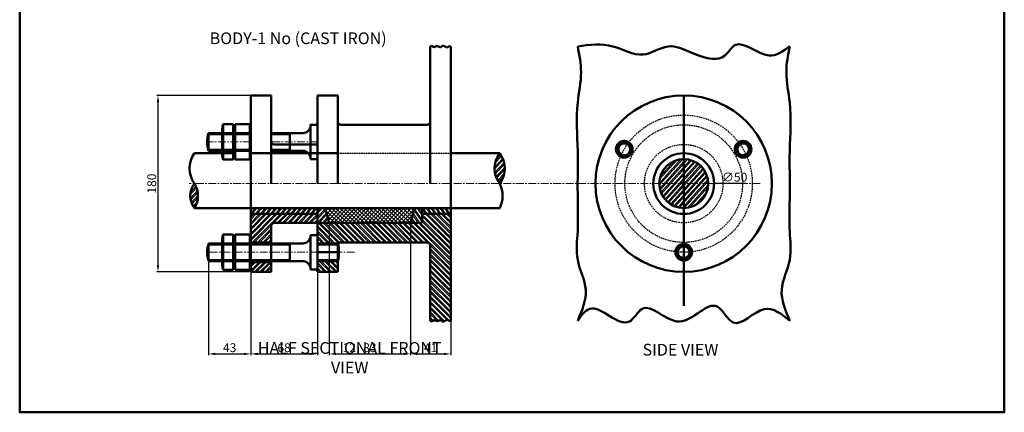
# Model space of a CAD drawing. Units: millimetres. Extents: x -98 to 907, y -783 to 313.
# Tile 1 of 3: x -98 to 907, y -783 to -383. Entities that reach past the tile are written whole.
import ezdxf

# ---------------------------------------------------------------- set-up
doc = ezdxf.new("R2010")
doc.units = ezdxf.units.MM
doc.header["$LTSCALE"] = 0.5
doc.linetypes.add('CENTER', pattern=[50.8, 31.75, -6.35, 6.35, -6.35])
doc.linetypes.add('HIDDEN', pattern=[9.525, 6.35, -3.175])
for name, color, linetype, lineweight in [('M-CNTR', 1, 'CENTER', 18), ('M-DIMS', 2, 'Continuous', 25), ('M-HATC', 8, 'Continuous', 18), ('M-HIDN', 4, 'HIDDEN', 25), ('M-OUTL', 7, 'Continuous', 50), ('M-TEXT', 3, 'Continuous', 25)]:
    doc.layers.add(name, color=color, linetype=linetype, lineweight=lineweight)
doc.styles.get("Standard").update_dxf_attribs({"font": 'arial.ttf'})
doc.dimstyles.new('ISO-25', dxfattribs={"dimtxt": 9, "dimasz": 7, "dimexe": 1.25, "dimexo": 0.625, "dimtad": 1, "dimtoh": 1, "dimtxsty": 'Standard', "dimcen": 2.5, "dimadec": 0, "dimazin": 0, "dimtfac": 1, "dimtofl": 0, "dimtmove": 0, "dimatfit": 3, "dimfxl": 1, "dimarcsym": 0})
pattern_1 = [(228, (1051.4906, -935.3726), (2.831382, -2.549388), []), (228, (1049.697, -935.4666), (2.831382, -2.549388), [])]

# ---------------------------------------------------------------- blocks, each defined once
blk = doc.blocks.new('NUT-HEX')
at = {"ltscale": 0.5}
for p, q in [((0, 16), (36, 16)), ((0, 8.5), (0, 16)), ((9, 8.5), (9, 17)), ((27, 17), (27, 8.5)), ((36, 16), (36, 8.5)), ((0, 1), (0, 8.5)), ((36, 1), (0, 1)), ((9, 1), (9, 8.5)), ((27, 8.5), (27, 1)), ((36, 8.5), (36, 1))]:
    blk.add_line(p, q, dxfattribs=at)
for centre, radius, start, end in [((4.5, 6.4), 10.6, 64.8152, 115.1848), ((18, -24), 41, 77.3196, 102.6804), ((31.5, 6.5), 10.6, 64.7565, 115.2435), ((4.5, 10.6), 10.6, 244.8152, 295.1848), ((18, 41), 41, 257.3196, 282.6804), ((31.5, 10.6), 10.6, 244.7565, 295.2435)]:
    blk.add_arc(centre, radius, start, end, dxfattribs=at)
blk = doc.blocks.new('STUD')
at = {"ltscale": 0.5}
for p, q in [((595.5, 113.7), (595.5, 78.7)), ((602.5, 113.7), (595.5, 113.7)), ((602.5, 78.7), (602.5, 113.7)), ((491.5, 105.2), (587.5, 105.2)), ((491.5, 87.2), (491.5, 105.2)), ((587.5, 87.2), (491.5, 87.2)), ((595.5, 78.7), (602.5, 78.7))]:
    blk.add_line(p, q, dxfattribs=at)
for centre, radius, start, end in [((587.5, 113.2), 8, 270, 0), ((517.6, 96.2), 27.6, 160.9887, 199.0113), ((587.5, 79.2), 8, 0, 90)]:
    blk.add_arc(centre, radius, start, end, dxfattribs=at)
blk = doc.blocks.new('*D41')
at = {"layer": 'Defpoints', "color": 0, "ltscale": 0.5, "transparency": 16777216}
for p in [(137.7, -639.8), (205.7, -639.8), (205.7, -723.6)]:
    blk.add_point(p, dxfattribs=at)
at = {"layer": 'M-DIMS', "color": 0, "lineweight": -2, "ltscale": 0.5, "transparency": 16777216}
for p, q in [((137.7, -640.5), (137.7, -724.8)), ((205.7, -640.5), (205.7, -724.8)), ((144.7, -723.6), (198.7, -723.6))]:
    blk.add_line(p, q, dxfattribs=at)
at = {"layer": 'M-DIMS', "color": 0, "ltscale": 0.5, "transparency": 16777216}
for points in [[(144.7, -722.4), (144.7, -724.8), (137.7, -723.6)], [(198.7, -722.4), (198.7, -724.8), (205.7, -723.6)]]:
    blk.add_solid(points, dxfattribs=at)
at = {"layer": 'M-DIMS', "color": 0, "ltscale": 0.5, "transparency": 16777216, "insert": (171.7, -718.4), "char_height": 9, "attachment_point": 5}
blk.add_mtext('68', dxfattribs=at)
blk = doc.blocks.new('*D42')
at = {"layer": 'Defpoints', "color": 0, "ltscale": 0.5, "transparency": 16777216}
for p in [(205.7, -589.8), (217.7, -589.8), (217.7, -723.6)]:
    blk.add_point(p, dxfattribs=at)
at = {"layer": 'M-DIMS', "color": 0, "lineweight": -2, "ltscale": 0.5, "transparency": 16777216}
for p, q in [((205.7, -590.5), (205.7, -724.8)), ((217.7, -590.5), (217.7, -724.8)), ((198.7, -723.6), (191.7, -723.6)), ((224.7, -723.6), (244.9, -723.6))]:
    blk.add_line(p, q, dxfattribs=at)
at = {"layer": 'M-DIMS', "color": 0, "ltscale": 0.5, "transparency": 16777216}
for points in [[(198.7, -722.4), (198.7, -724.8), (205.7, -723.6)], [(224.7, -722.4), (224.7, -724.8), (217.7, -723.6)]]:
    blk.add_solid(points, dxfattribs=at)
at = {"layer": 'M-DIMS', "color": 0, "ltscale": 0.5, "transparency": 16777216, "insert": (238.3, -718.4), "char_height": 9, "attachment_point": 5}
blk.add_mtext('12', dxfattribs=at)
blk = doc.blocks.new('*D43')
at = {"layer": 'Defpoints', "color": 0, "ltscale": 0.5, "transparency": 16777216}
for p in [(217.7, -589.8), (300.7, -589.8), (300.7, -723.6)]:
    blk.add_point(p, dxfattribs=at)
at = {"layer": 'M-DIMS', "color": 0, "lineweight": -2, "ltscale": 0.5, "transparency": 16777216}
for p, q in [((217.7, -590.5), (217.7, -724.8)), ((300.7, -590.5), (300.7, -724.8)), ((224.7, -723.6), (293.7, -723.6))]:
    blk.add_line(p, q, dxfattribs=at)
at = {"layer": 'M-DIMS', "color": 0, "ltscale": 0.5, "transparency": 16777216}
for points in [[(224.7, -722.4), (224.7, -724.8), (217.7, -723.6)], [(293.7, -722.4), (293.7, -724.8), (300.7, -723.6)]]:
    blk.add_solid(points, dxfattribs=at)
at = {"layer": 'M-DIMS', "color": 0, "ltscale": 0.5, "transparency": 16777216, "insert": (259.2, -718.4), "char_height": 9, "attachment_point": 5}
blk.add_mtext('83', dxfattribs=at)
blk = doc.blocks.new('*D44')
at = {"layer": 'Defpoints', "color": 0, "ltscale": 0.5, "transparency": 16777216}
for p in [(341.7, -580.8), (300.7, -589.8), (341.7, -723.6)]:
    blk.add_point(p, dxfattribs=at)
at = {"layer": 'M-DIMS', "color": 0, "lineweight": -2, "ltscale": 0.5, "transparency": 16777216}
for p, q in [((341.7, -581.5), (341.7, -724.8)), ((300.7, -590.5), (300.7, -724.8)), ((307.7, -723.6), (334.7, -723.6))]:
    blk.add_line(p, q, dxfattribs=at)
at = {"layer": 'M-DIMS', "color": 0, "ltscale": 0.5, "transparency": 16777216}
for points in [[(307.7, -722.4), (307.7, -724.8), (300.7, -723.6)], [(334.7, -722.4), (334.7, -724.8), (341.7, -723.6)]]:
    blk.add_solid(points, dxfattribs=at)
at = {"layer": 'M-DIMS', "color": 0, "ltscale": 0.5, "transparency": 16777216, "insert": (321.2, -718.4), "char_height": 9, "attachment_point": 5}
blk.add_mtext('41', dxfattribs=at)
blk = doc.blocks.new('*D45')
at = {"layer": 'Defpoints', "color": 0, "ltscale": 0.5, "transparency": 16777216}
for p in [(94.7, -628.8), (137.7, -639.8), (137.7, -723.6)]:
    blk.add_point(p, dxfattribs=at)
at = {"layer": 'M-DIMS', "color": 0, "lineweight": -2, "ltscale": 0.5, "transparency": 16777216}
for p, q in [((94.7, -629.5), (94.7, -724.8)), ((137.7, -640.5), (137.7, -724.8)), ((101.7, -723.6), (130.7, -723.6))]:
    blk.add_line(p, q, dxfattribs=at)
at = {"layer": 'M-DIMS', "color": 0, "ltscale": 0.5, "transparency": 16777216}
for points in [[(101.7, -722.4), (101.7, -724.8), (94.7, -723.6)], [(130.7, -722.4), (130.7, -724.8), (137.7, -723.6)]]:
    blk.add_solid(points, dxfattribs=at)
at = {"layer": 'M-DIMS', "color": 0, "ltscale": 0.5, "transparency": 16777216, "insert": (116.2, -718.4), "char_height": 9, "attachment_point": 5}
blk.add_mtext('43', dxfattribs=at)
blk = doc.blocks.new('*D46')
at = {"layer": 'Defpoints', "color": 0, "ltscale": 0.5, "transparency": 16777216}
for p in [(137.7, -459.8), (43, -639.8), (137.7, -639.8)]:
    blk.add_point(p, dxfattribs=at)
at = {"layer": 'M-DIMS', "color": 0, "lineweight": -2, "ltscale": 0.5, "transparency": 16777216}
for p, q in [((137, -459.8), (41.7, -459.8)), ((43, -466.8), (43, -632.8)), ((137, -639.8), (41.7, -639.8))]:
    blk.add_line(p, q, dxfattribs=at)
at = {"layer": 'M-DIMS', "color": 0, "ltscale": 0.5, "transparency": 16777216}
for points in [[(41.8, -466.8), (44.2, -466.8), (43, -459.8)], [(41.8, -632.8), (44.2, -632.8), (43, -639.8)]]:
    blk.add_solid(points, dxfattribs=at)
at = {"layer": 'M-DIMS', "color": 0, "ltscale": 0.5, "transparency": 16777216, "insert": (37.8, -549.8), "char_height": 9, "attachment_point": 5, "rotation": 90}
blk.add_mtext('180', dxfattribs=at)
blk = doc.blocks.new('*D54')
at = {"layer": 'Defpoints', "color": 0, "ltscale": 0.5, "transparency": 16777216}
for p in [(554.5, -549.8), (604.5, -549.8)]:
    blk.add_point(p, dxfattribs=at)
at = {"layer": 'M-DIMS', "color": 0, "lineweight": -2, "ltscale": 0.5, "transparency": 16777216}
for p, q in [((577, -549.8), (582, -549.8)), ((579.5, -552.3), (579.5, -547.3)), ((619.5, -549.8), (611.5, -549.8)), ((642.7, -549.8), (619.5, -549.8))]:
    blk.add_line(p, q, dxfattribs=at)
at = {"layer": 'M-DIMS', "color": 0, "ltscale": 0.5, "transparency": 16777216}
blk.add_solid([(611.5, -548.7), (611.5, -551), (604.5, -549.8)], dxfattribs=at)
at = {"layer": 'M-DIMS', "color": 0, "ltscale": 0.5, "transparency": 16777216, "insert": (631.4, -544.4), "char_height": 9, "attachment_point": 5}
blk.add_mtext('∅50', dxfattribs=at)

msp = doc.modelspace()

# ---------------------------------------------------------------- hatches: boundary and pattern name
at = {"layer": 'M-HATC', "ltscale": 0.5}
h = msp.add_hatch(dxfattribs=at)
h.set_pattern_fill('ANSI32', color=256, scale=0.4, angle=363)
h.set_pattern_definition([(48, (783.4996, -819.342), (-2.831382, 2.549388), []), (48, (785.293, -819.248), (-2.831382, 2.549388), [])])
h.paths.add_polyline_path([(137.6706, -580.8393), (205.6706, -580.8393), (205.6706, -589.8393), (217.6706, -589.8393), (213.6514, -574.8393), (137.6706, -574.8393)])
edge = h.paths.add_edge_path()
edge.add_arc((127.101, -520.8393), 10.5748, 358.1956679, 361.8043321)
edge.add_line((137.6706, -520.5063), (137.6706, -521.1722))
h = msp.add_hatch(dxfattribs=at)
h.set_pattern_fill('ANSI32', color=256, scale=0.4, angle=183)
h.set_pattern_definition(pattern_1)
h.paths.add_polyline_path([(391.6706, -518.8393, 0.336981318), (391.6706, -549.8393, 0.336981318)])
h = msp.add_hatch(dxfattribs=at)
h.set_pattern_fill('ANSI32', color=256, scale=0.4, angle=183)
h.paths.add_polyline_path([(579.4617, -524.8393, 0.414213562), (554.4617, -549.8393), (579.4617, -549.8393)])
h.paths.add_polyline_path([(579.4617, -524.8393), (579.4617, -549.8393), (604.4617, -549.8393, 0.414213562)])
h.paths.add_polyline_path([(604.4617, -549.8393), (579.4617, -549.8393), (579.4617, -574.8393, 0.414213562)])
h.paths.add_polyline_path([(579.4617, -549.8393), (554.4617, -549.8393, 0.414213562), (579.4617, -574.8393)])
h = msp.add_hatch(dxfattribs=at)
h.set_pattern_fill('ANSI32', color=256, scale=0.4, angle=183)
h.set_pattern_definition(pattern_1)
h.paths.add_polyline_path([(80.2178, -574.8393, 0.290271984), (80.2178, -549.8393, 0.335154212)])
h = msp.add_hatch(dxfattribs=at)
h.set_pattern_fill('ANSI32', color=256, scale=0.4)
h.set_pattern_definition([(45, (37.2156, -636.4595), (-2.69408, 2.69408), []), (45, (39.0116, -636.4595), (-2.69408, 2.69408), [])])
h.paths.add_polyline_path([(137.6706, -629.8393), (137.6706, -639.8393), (158.6706, -639.8393), (158.6706, -629.8393)])
h.paths.add_polyline_path([(137.6706, -609.8393), (158.6706, -609.8393), (158.6706, -592.8393, -0.414213562), (161.6706, -589.8393), (205.6706, -589.8393), (205.6706, -580.8393), (137.6706, -580.8393)])
h = msp.add_hatch(dxfattribs=at)
h.set_pattern_fill('ANSI32', color=256, scale=0.4, angle=90)
h.set_pattern_definition([(135, (72.0148, -304.6603), (-2.694077, -2.694077), []), (135, (72.0148, -302.8642), (-2.694077, -2.694077), [])])
edge = h.paths.add_edge_path()
edge.add_line((205.6706, -589.8393), (205.6706, -610.8393))
edge.add_line((205.6706, -610.8393), (226.6706, -610.8393))
edge.add_arc((227.6706, -610.8393), 1, 90, 180, ccw=False)
edge.add_line((227.6706, -609.8393), (317.6706, -609.8393))
edge.add_arc((317.6706, -612.8393), 3, 0, 90, ccw=False)
edge.add_line((320.6706, -612.8393), (320.6706, -689.8393))
edge.add_spline(control_points=[(320.6706, -689.8393), (321.733, -690.1461), (323.0212, -690.5181), (324.0986, -689.0345), (326.0649, -689.3768), (328.3511, -691.1881), (331.5052, -687.656), (333.7152, -692.8045), (337.7716, -687.356), (339.66, -690.1085), (340.8232, -689.9527), (341.6706, -689.8393)], knot_values=[0, 0, 0, 0, 2.795650421, 3.389792184, 5.125359391, 7.794235645, 11.48125794, 13.701506228, 19.514089341, 20.367966623, 22.658878867, 22.658878867, 22.658878867, 22.658878867], degree=3, periodic=0)
edge.add_line((341.6706, -689.8393), (341.6706, -580.8393))
edge.add_line((341.6706, -580.8393), (312.6706, -580.8393))
edge.add_line((312.6706, -580.8393), (312.6706, -589.8393))
edge.add_line((312.6706, -589.8393), (205.6706, -589.8393))
h.paths.add_polyline_path([(205.6706, -628.8393), (205.6706, -639.8393), (226.6706, -639.8393), (226.6706, -628.8393)], flags=17)
h = msp.add_hatch(dxfattribs=at)
h.set_pattern_fill('ANSI37', color=256, scale=0.9, angle=183)
h.paths.add_polyline_path([(304.6898, -574.8393), (213.6514, -574.8393), (217.6706, -589.8393), (300.6706, -589.8393)])
h = msp.add_hatch(dxfattribs=at)
h.set_pattern_fill('ANSI32', color=256, scale=0.4, angle=80)
h.set_pattern_definition([(125, (-265.1583, -447.9016), (-3.12097, -2.185326), []), (125, (-264.8465, -446.1328), (-3.12097, -2.185326), [])])
h.paths.add_polyline_path([(312.6706, -580.8393), (341.6706, -580.8393), (341.6706, -574.8393), (304.6898, -574.8393), (300.6706, -589.8393), (312.6706, -589.8393)])

# ---------------------------------------------------------------- linework, layer by layer
at = {"layer": 'M-CNTR', "ltscale": 0.5}
for p, q in [((137.6706, -507.3393), (94.6706, -507.3393)), ((205.6706, -507.3393), (158.7126, -507.3393)), ((229.3888, -549.8393), (74.9893, -549.8393)), ((205.6706, -549.8393), (341.6706, -549.8393)), ((344.7631, -549.8393), (658.4786, -549.8393)), ((243.6184, -619.8393), (94.6706, -619.8393))]:
    msp.add_line(p, q, dxfattribs=at)
at = {"layer": 'M-HIDN'}
msp.add_line((137.6706, -518.8393), (205.6706, -518.8393), dxfattribs=at)
at = {"layer": 'M-HIDN', "ltscale": 0.5}
msp.add_line((226.6706, -518.8393), (341.6706, -518.8393), dxfattribs=at)
for radius in [70, 60, 40]:
    msp.add_circle((579.4617, -549.8393), radius, dxfattribs=at)
at = {"layer": 'M-OUTL', "ltscale": 0.5}
for p, q in [((320.6706, -486.8393), (320.6706, -409.8393)), ((341.6706, -409.8393), (341.6706, -689.8393)), ((205.6706, -459.8393), (205.6706, -549.8393)), ((226.6706, -459.8393), (205.6706, -459.8393)), ((226.6706, -549.8393), (226.6706, -459.8393)), ((579.4617, -459.8393), (579.4617, -674.4759)), ((229.6706, -489.8393), (317.6706, -489.8393)), ((320.6706, -549.8393), (320.6706, -486.8393)), ((94.6706, -498.3393), (137.6706, -498.3393)), ((94.6706, -499.3393), (137.6706, -499.3393)), ((108.6706, -521.1722), (108.6706, -493.4372)), ((120.6706, -521.1722), (120.6706, -493.4372)), ((120.6706, -521.1722), (120.6706, -493.4372)), ((137.6706, -521.1722), (137.6706, -493.4372)), ((158.6706, -498.3393), (190.6706, -498.3393)), ((158.6706, -499.3393), (177.6706, -499.3393)), ((177.6706, -516.3393), (177.6706, -498.3393)), ((226.6706, -516.3393), (226.6706, -498.3393)), ((205.6706, -518.8393), (205.6706, -509.8393)), ((121.6706, -518.8393), (80.2178, -518.8393)), ((137.6706, -515.3393), (94.6706, -515.3393)), ((226.6706, -518.8393), (136.6706, -518.8393)), ((137.6706, -580.8393), (137.6706, -518.8393)), ((137.6706, -518.8393), (205.6706, -518.8393)), ((158.6706, -515.3393), (177.6706, -515.3393)), ((158.6706, -516.3393), (190.6706, -516.3393)), ((158.6706, -518.8393), (158.6706, -549.8393)), ((341.6706, -518.8393), (341.6706, -580.8393)), ((341.6706, -518.8393), (391.6706, -518.8393)), ((579.4617, -516.5232), (579.4617, -606.1013)), ((198.6706, -524.8393), (205.6706, -524.8393)), ((80.2178, -574.8393), (391.6706, -574.8393)), ((137.6706, -574.8393), (213.6514, -574.8393)), ((137.6706, -580.8393), (205.6706, -580.8393)), ((205.6706, -574.8393), (205.6706, -639.8393)), ((205.6706, -580.8393), (205.6706, -589.8393)), ((213.6514, -574.8393), (217.6706, -589.8393)), ((304.6898, -574.8393), (300.6706, -589.8393)), ((341.6706, -574.8393), (304.6898, -574.8393)), ((312.6706, -589.8393), (312.6706, -574.8393)), ((312.6706, -580.8393), (341.6706, -580.8393)), ((341.6706, -580.8393), (312.6706, -580.8393)), ((312.6706, -580.8393), (312.6706, -589.8393)), ((205.6706, -589.8393), (312.6706, -589.8393)), ((205.6706, -589.8393), (217.6706, -589.8393)), ((312.6706, -589.8393), (300.6706, -589.8393)), ((94.6706, -611.8393), (177.6706, -611.8393)), ((108.6706, -633.6377), (108.6706, -605.9027)), ((120.6706, -633.6377), (120.6706, -605.9027)), ((120.6706, -633.6722), (120.6706, -605.9372)), ((137.6706, -633.6722), (137.6706, -605.9372)), ((158.6706, -609.8393), (137.6706, -609.8393)), ((177.6706, -628.8393), (177.6706, -610.8393)), ((205.6706, -610.8393), (226.6706, -610.8393)), ((205.6706, -610.8393), (226.6706, -610.8393)), ((205.6706, -611.8393), (226.6706, -611.8393)), ((226.6706, -639.8393), (226.6706, -610.8393)), ((226.6706, -628.8393), (226.6706, -610.8393)), ((227.6706, -609.8393), (317.6706, -609.8393)), ((320.6706, -689.8393), (320.6706, -612.8393)), ((205.6706, -619.8393), (226.6706, -619.8393)), ((177.6706, -627.8393), (94.6706, -627.8393)), ((158.6706, -629.8393), (137.6706, -629.8393)), ((226.6706, -627.8393), (205.6706, -627.8393)), ((205.6706, -628.8393), (226.6706, -628.8393)), ((226.6706, -628.8393), (205.6706, -628.8393)), ((205.6706, -639.8393), (226.6706, -639.8393))]:
    msp.add_line(p, q, dxfattribs=at)
at = {"layer": 'M-OUTL'}
for p, q in [((137.6706, -459.8393), (137.6706, -639.8393)), ((158.6706, -459.8393), (137.6706, -459.8393)), ((158.6706, -518.8393), (158.6706, -459.8393)), ((205.6706, -509.8393), (161.6706, -509.8393)), ((205.6706, -549.8393), (205.6706, -509.8393)), ((137.6706, -580.8393), (205.6706, -580.8393)), ((205.6706, -589.8393), (205.6706, -574.8393)), ((205.6706, -589.8393), (161.6706, -589.8393)), ((158.6706, -639.8393), (158.6706, -592.8393)), ((137.6706, -639.8393), (158.6706, -639.8393))]:
    msp.add_line(p, q, dxfattribs=at)
at = {"layer": 'M-OUTL', "ltscale": 0.5}
for points in [[(-98.0885, 312.8308), (906.5931, 312.8308), (906.5931, -783.1771), (-98.0885, -783.1771)], [(198.6706, -524.8393), (205.6706, -524.8393), (205.6706, -489.8393), (198.6706, -489.8393)], [(518.8399, -506.3393), (511.4787, -510.5893), (511.4787, -519.0893), (518.8399, -523.3393), (526.2011, -519.0893), (526.2011, -510.5893)], [(640.0834, -506.3393), (632.7222, -510.5893), (632.7222, -519.0893), (640.0834, -523.3393), (647.4446, -519.0893), (647.4446, -510.5893)], [(226.6706, -516.3393), (226.6706, -516.3393)], [(579.4617, -611.3393), (572.1004, -615.5893), (572.1004, -624.0893), (579.4617, -628.3393), (586.8229, -624.0893), (586.8229, -615.5893)]]:
    msp.add_lwpolyline(points, close=True, dxfattribs=at)
for points in [[(109.6706, -525.3393, -0.223387372), (109.6706, -516.3393, -0.111111111), (109.6706, -498.3393, -0.223925015), (109.6706, -489.3393), (109.6706, -525.3393), (114.6706, -525.3393), (119.6706, -525.3393, 0.223387372), (119.6706, -516.3393, 0.111111111), (119.6706, -498.3393, 0.223925015), (119.6706, -489.3393), (119.6706, -525.3393)], [(198.6706, -524.3393, 0.414213562), (190.6706, -516.3393), (177.6706, -516.3393)], [(109.6706, -637.8047, -0.223387372), (109.6706, -628.8047, -0.111111111), (109.6706, -610.8047, -0.223925015), (109.6706, -601.8047), (109.6706, -637.8047), (114.6706, -637.8047), (119.6706, -637.8047, 0.223387372), (119.6706, -628.8047, 0.111111111), (119.6706, -610.8047, 0.223925015), (119.6706, -601.8047), (119.6706, -637.8047)]]:
    msp.add_lwpolyline(points, format="xyb", dxfattribs=at)
for points in [[(109.6706, -489.3393), (114.6706, -489.3393), (119.6706, -489.3393)], [(108.6706, -498.3393), (114.6706, -498.3393), (119.6706, -498.3393)], [(137.6706, -516.3393), (94.6706, -516.3393)], [(119.6706, -516.3393), (114.6706, -516.3393), (108.6706, -516.3393)], [(109.6706, -601.8047), (114.6706, -601.8047), (119.6706, -601.8047)], [(108.6706, -610.8047), (114.6706, -610.8047), (119.6706, -610.8047)], [(119.6706, -628.8047), (114.6706, -628.8047), (108.6706, -628.8047)]]:
    msp.add_lwpolyline(points, dxfattribs=at)
msp.add_lwpolyline([(94.6706, -498.3393, 0.167444228), (94.6706, -516.3393)], format="xyb", close=True, dxfattribs=at)
for centre, radius in [((579.4617, -549.8393), 90), ((518.8399, -514.8393), 8.5), ((518.8399, -514.8393), 6), ((640.0834, -514.8393), 8.5), ((640.0834, -514.8393), 6), ((579.4617, -549.8393), 31), ((579.4617, -549.8393), 25), ((579.4617, -619.8393), 8.5), ((579.4617, -619.8393), 6)]:
    msp.add_circle(centre, radius, dxfattribs=at)
for centre, radius, start, end in [((190.6706, -490.3393), 8, 270, 0), ((229.6706, -486.8393), 3, 180, 270), ((317.6706, -486.8393), 3, 270, 0), ((102.0453, -534.3393), 26.7711, 144.6210031, 215.3789969), ((412.0573, -534.3393), 25.6099, 142.7542896, 217.2457104), ((371.2839, -534.3393), 25.6099, 322.7542896, 37.2457104), ((96.7712, -562.3393), 20.7428, 142.9424135, 217.0575865), ((60.5004, -562.3393), 23.3457, 327.6269348, 32.3730652), ((366.615, -562.3393), 28.0006, 333.4858158, 26.5141842), ((227.6706, -610.8393), 1, 90, 180), ((184.873, -619.8393), 42.7556, 347.848408, 12.151592), ((317.6706, -612.8393), 3, 0, 90)]:
    msp.add_arc(centre, radius, start, end, dxfattribs=at)
at = {"layer": 'M-OUTL'}
for centre, start, end in [((161.6706, -506.8393), 180, 270), ((161.6706, -592.8393), 90, 180)]:
    msp.add_arc(centre, 3, start, end, dxfattribs=at)
at = {"layer": 'M-OUTL', "ltscale": 0.5}
for points, knots in [([(320.6706, -409.8393), (321.733, -409.5325), (323.0212, -409.1605), (324.0986, -410.644), (326.0649, -410.3018), (328.3511, -408.4905), (331.5052, -412.0226), (333.7152, -406.8741), (337.7716, -412.3226), (339.66, -409.57), (340.8232, -409.7258), (341.6706, -409.8393)], [0, 0, 0, 0, 2.795650421, 3.389792184, 5.125359391, 7.794235645, 11.48125794, 13.701506228, 19.514089341, 20.367966623, 22.658878867, 22.658878867, 22.658878867, 22.658878867]), ([(471.2594, -409.8393), (472.9993, -418.6452), (476.7609, -437.6832), (468.6183, -473.0458), (472.1256, -514.5716), (470.7131, -558.4758), (472.3883, -595.4294), (468.125, -628.8035), (484.5714, -658.4249), (475.7338, -679.2803), (471.2594, -689.8393)], [0, 0, 0, 0, 26.651305799, 57.619250961, 106.866574805, 150.942750145, 189.282947528, 218.107151479, 249.931939448, 282.568373609, 282.568373609, 282.568373609, 282.568373609]), ([(471.2594, -409.8393), (483.3765, -408.2455), (506.2069, -405.2425), (536.3433, -424.7222), (565.8517, -403.1825), (591.4421, -420.2752), (620.0544, -425.7232), (634.9282, -397.5617), (663.4253, -427.5075), (680.8863, -414.7797), (687.6639, -409.8393)], [0, 0, 0, 0, 36.008703464, 67.845945229, 94.595179736, 128.047433648, 153.491524271, 168.674800281, 205.05951054, 228.142437657, 228.142437657, 228.142437657, 228.142437657]), ([(687.6639, -409.8393), (685.924, -418.6452), (682.1624, -437.6832), (690.305, -473.0458), (686.7977, -514.5716), (688.2103, -558.4758), (686.535, -595.4294), (690.7983, -628.8035), (674.3519, -658.4249), (683.1895, -679.2803), (687.6639, -689.8393)], [0, 0, 0, 0, 26.651305799, 57.619250961, 106.866574805, 150.942750145, 189.282947528, 218.107151479, 249.931939448, 282.568373609, 282.568373609, 282.568373609, 282.568373609]), ([(471.2594, -689.8393), (475.0366, -684.3066), (488.0084, -665.3064), (520.3204, -705.8045), (540.2929, -663.5593), (575.9297, -710.097), (611.0679, -658.6563), (630.9282, -705.3874), (660.4877, -667.6378), (679.1756, -682.9048), (687.6639, -689.8393)], [0, 0, 0, 0, 17.45434219, 59.941520252, 77.823004087, 118.322250159, 159.712555172, 182.805932108, 217.271917639, 245.955091385, 245.955091385, 245.955091385, 245.955091385]), ([(320.6706, -689.8393), (321.733, -690.1461), (323.0212, -690.5181), (324.0986, -689.0345), (326.0649, -689.3768), (328.3511, -691.1881), (331.5052, -687.656), (333.7152, -692.8045), (337.7716, -687.356), (339.66, -690.1085), (340.8232, -689.9527), (341.6706, -689.8393)], [0, 0, 0, 0, 2.795650421, 3.389792184, 5.125359391, 7.794235645, 11.48125794, 13.701506228, 19.514089341, 20.367966623, 22.658878867, 22.658878867, 22.658878867, 22.658878867])]:
    msp.add_open_spline(points, degree=3, knots=knots, dxfattribs=at)

# ---------------------------------------------------------------- block references
at = {"layer": 'M-OUTL'}
for p, rotation in [((137.678, -525.3394), 90.0000000000003), ((137.678, -637.8394), 90.00000000000018)]:
    msp.add_blockref('NUT-HEX', p, dxfattribs=dict(at, rotation=rotation))
msp.add_blockref('STUD', (-396.7801, -716.0516), dxfattribs=at)

# ---------------------------------------------------------------- texts
at = {"layer": 'M-TEXT', "ltscale": 0.5, "char_height": 12, "attachment_point": 1}
for s, insert in [('\\pxqc;BODY-1 No (CAST IRON)', (86.165, -395.5434)), ('\\pxqc;HALF SECTIONAL FRONT VIEW', (138.7379, -711.5158)), ('\\pxqc;SIDE VIEW', (476.267, -713.317))]:
    msp.add_mtext_dynamic_manual_height_columns(s, width=199.843565, gutter_width=12.5, heights=[0], dxfattribs=dict(at, insert=insert))

# ---------------------------------------------------------------- dimensions: what is measured, and where the dimension line sits
at = {"layer": 'M-DIMS', "ltscale": 0.5}
dim = msp.add_linear_dim(base=(42.9893, -639.8393), p1=(137.6706, -459.8393), p2=(137.6706, -639.8393), angle=90, dimstyle='ISO-25', override={"dimdec": 0, "dimlfac": 1, "dimrnd": 0, "dimzin": 0, "dimdsep": 46, "dimlunit": 2}, dxfattribs=at)
dim.commit()
dim.dimension.update_dxf_attribs({"geometry": '*D46', "text_midpoint": (37.7692, -549.8393)})
dim = msp.add_diameter_dim_2p(p1=(554.4617, -549.8396), p2=(604.4617, -549.839), dimstyle='ISO-25', override={"dimdec": 0, "dimlfac": 1, "dimrnd": 0, "dimzin": 0, "dimdsep": 46, "dimlunit": 2}, dxfattribs=at)
dim.commit()
dim.dimension.update_dxf_attribs({"geometry": '*D54', "text_midpoint": (619.4617, -549.8388), "dimtype": 163})
for base, p1, p2, picture, middle in [((341.6706, -723.5852), (300.6706, -589.8393), (341.6706, -580.8393), '*D44', (321.1706, -718.4418)), ((217.6706, -723.5852), (205.6706, -589.8393), (217.6706, -589.8393), '*D42', (238.2721, -718.4418)), ((300.6706, -723.5852), (217.6706, -589.8393), (300.6706, -589.8393), '*D43', (259.1706, -718.362)), ((137.6706, -723.5852), (94.6706, -628.8393), (137.6706, -639.8393), '*D45', (116.1706, -718.362)), ((205.6706, -723.5852), (137.6706, -639.8393), (205.6706, -639.8393), '*D41', (171.6706, -718.365))]:
    dim = msp.add_linear_dim(base=base, p1=p1, p2=p2, dimstyle='ISO-25', override={"dimdec": 0, "dimlfac": 1, "dimrnd": 0, "dimzin": 0, "dimdsep": 46, "dimlunit": 2}, dxfattribs=at)
    dim.commit()
    dim.dimension.update_dxf_attribs({"geometry": picture, "text_midpoint": middle})

doc.saveas('drawing.dxf')
